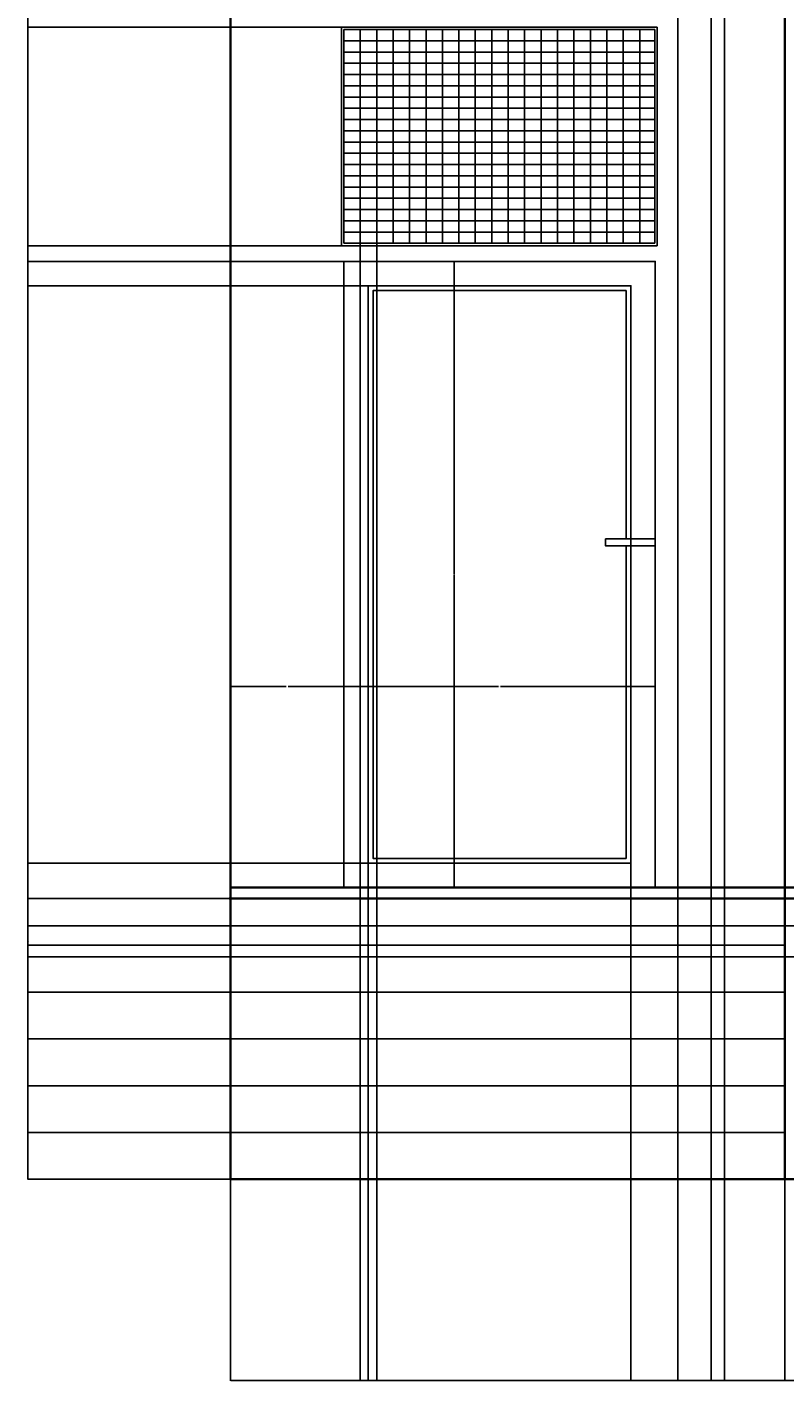
# Model space of a CAD drawing. Units: inches. Extents: x 1231 to 2151, y 481 to 2277.
# Tile 1 of 7: x 1231 to 1542, y 481 to 1038. Entities that reach past the tile are written whole.
import ezdxf

# ---------------------------------------------------------------- set-up
doc = ezdxf.new("R2010")
doc.units = ezdxf.units.IN
doc.header["$MEASUREMENT"] = 0
for name, color, linetype, lineweight in [('A-ANNO-DIMS', 2, 'Continuous', 18), ('A-DOOR', 4, 'Continuous', 25), ('A-ELEV', 7, 'Continuous', 35), ('A-FLOR-STRS', 2, 'Continuous', 25), ('A-GLAZ', 3, 'Continuous', 25)]:
    doc.layers.add(name, color=color, linetype=linetype, lineweight=lineweight)
doc.styles.get("Standard").update_dxf_attribs({"font": 'arial.ttf'})
doc.dimstyles.get("Standard").update_dxf_attribs({"dimtxt": 0.18, "dimasz": 0.18, "dimexe": 0.18, "dimexo": 0.0625, "dimgap": 0.09, "dimtad": 0, "dimtih": 1, "dimtoh": 1, "dimdec": 0, "dimzin": 0, "dimdsep": 46, "dimlunit": 3, "dimtxsty": 'Standard', "dimcen": 0.09, "dimadec": 0, "dimazin": 0, "dimtfac": 1, "dimtdec": 0, "dimtofl": 0, "dimtmove": 0, "dimatfit": 3, "dimfxl": 1, "dimtolj": 1, "dimtzin": 0, "dimarcsym": 0})

# ---------------------------------------------------------------- blocks, each defined once
blk = doc.blocks.new('*D1')
at = {"layer": 'A-ANNO-DIMS', "color": 0, "lineweight": -2, "transparency": 16777216}
for p, q in [((1314.24, 563.63), (1314.24, 480.76)), ((2067.47, 563.63), (2067.47, 480.76)), ((1314.42, 480.94), (1690.47, 480.94)), ((2067.29, 480.94), (1691.25, 480.94))]:
    blk.add_line(p, q, dxfattribs=at)
at = {"layer": 'A-ANNO-DIMS', "color": 0, "transparency": 16777216}
for points in [[(1314.42, 480.97), (1314.42, 480.91), (1314.24, 480.94)], [(2067.29, 480.97), (2067.29, 480.91), (2067.47, 480.94)]]:
    blk.add_solid(points, dxfattribs=at)
at = {"layer": 'Defpoints', "color": 0, "transparency": 16777216}
for p in [(1314.24, 563.69), (2067.47, 563.69), (2067.47, 480.94)]:
    blk.add_point(p, dxfattribs=at)
at = {"layer": 'A-ANNO-DIMS', "color": 0, "transparency": 16777216, "insert": (1690.86, 480.94), "char_height": 0.18, "attachment_point": 5}
blk.add_mtext('\\A1;753.2', dxfattribs=at)
blk = doc.blocks.new('*D2')
at = {"layer": 'A-ANNO-DIMS', "color": 0, "lineweight": -2, "transparency": 16777216}
for p, q in [((1314.18, 2193.78), (1230.78, 2193.78)), ((1230.96, 2193.6), (1230.96, 1378.92)), ((1230.96, 563.87), (1230.96, 1378.55)), ((1314.18, 563.69), (1230.78, 563.69))]:
    blk.add_line(p, q, dxfattribs=at)
at = {"layer": 'A-ANNO-DIMS', "color": 0, "transparency": 16777216}
for points in [[(1230.93, 2193.6), (1230.99, 2193.6), (1230.96, 2193.78)], [(1230.93, 563.87), (1230.99, 563.87), (1230.96, 563.69)]]:
    blk.add_solid(points, dxfattribs=at)
at = {"layer": 'Defpoints', "color": 0, "transparency": 16777216}
for p in [(1230.96, 2193.78), (1314.24, 2193.78), (1314.24, 563.69)]:
    blk.add_point(p, dxfattribs=at)
at = {"layer": 'A-ANNO-DIMS', "color": 0, "transparency": 16777216, "insert": (1230.96, 1378.74), "char_height": 0.18, "attachment_point": 5}
blk.add_mtext('\\A1;1630', dxfattribs=at)
blk = doc.blocks.new('*D29')
at = {"layer": 'A-ANNO-DIMS', "color": 0, "lineweight": -2, "transparency": 16777216}
for p, q in [((1314.24, 683.75), (1314.24, 766.62)), ((1314.42, 766.44), (1337.18, 766.44)), ((1360.73, 766.44), (1337.97, 766.44)), ((1360.91, 683.75), (1360.91, 766.62))]:
    blk.add_line(p, q, dxfattribs=at)
at = {"layer": 'A-ANNO-DIMS', "color": 0, "transparency": 16777216}
for points in [[(1314.42, 766.47), (1314.42, 766.41), (1314.24, 766.44)], [(1360.73, 766.47), (1360.73, 766.41), (1360.91, 766.44)]]:
    blk.add_solid(points, dxfattribs=at)
at = {"layer": 'Defpoints', "color": 0, "transparency": 16777216}
for p in [(1360.91, 766.44), (1314.24, 683.69), (1360.91, 683.69)]:
    blk.add_point(p, dxfattribs=at)
at = {"layer": 'A-ANNO-DIMS', "color": 0, "transparency": 16777216, "insert": (1337.57, 766.44), "char_height": 0.18, "attachment_point": 5}
blk.add_mtext('\\A1;46.67', dxfattribs=at)
blk = doc.blocks.new('*D30')
at = {"layer": 'A-ANNO-DIMS', "color": 0, "lineweight": -2, "transparency": 16777216}
for p, q in [((1360.91, 683.75), (1360.91, 766.62)), ((1361.09, 766.44), (1424.59, 766.44)), ((1488.84, 766.44), (1425.33, 766.44)), ((1489.02, 683.75), (1489.02, 766.62))]:
    blk.add_line(p, q, dxfattribs=at)
at = {"layer": 'A-ANNO-DIMS', "color": 0, "transparency": 16777216}
for points in [[(1361.09, 766.47), (1361.09, 766.41), (1360.91, 766.44)], [(1488.84, 766.47), (1488.84, 766.41), (1489.02, 766.44)]]:
    blk.add_solid(points, dxfattribs=at)
at = {"layer": 'Defpoints', "color": 0, "transparency": 16777216}
for p in [(1489.02, 766.44), (1360.91, 683.69), (1489.02, 683.69)]:
    blk.add_point(p, dxfattribs=at)
at = {"layer": 'A-ANNO-DIMS', "color": 0, "transparency": 16777216, "insert": (1424.96, 766.44), "char_height": 0.18, "attachment_point": 5}
blk.add_mtext('\\A1;128.1', dxfattribs=at)
blk = doc.blocks.new('*D31')
at = {"layer": 'A-ANNO-DIMS', "color": 0, "lineweight": -2, "transparency": 16777216}
for p, q in [((1488.95, 941.31), (1406.09, 941.31)), ((1406.27, 941.13), (1406.27, 812.68)), ((1406.27, 683.87), (1406.27, 812.32)), ((1488.95, 683.69), (1406.09, 683.69))]:
    blk.add_line(p, q, dxfattribs=at)
at = {"layer": 'A-ANNO-DIMS', "color": 0, "transparency": 16777216}
for points in [[(1406.24, 941.13), (1406.3, 941.13), (1406.27, 941.31)], [(1406.24, 683.87), (1406.3, 683.87), (1406.27, 683.69)]]:
    blk.add_solid(points, dxfattribs=at)
at = {"layer": 'Defpoints', "color": 0, "transparency": 16777216}
for p in [(1406.27, 941.31), (1489.02, 941.31), (1489.02, 683.69)]:
    blk.add_point(p, dxfattribs=at)
at = {"layer": 'A-ANNO-DIMS', "color": 0, "transparency": 16777216, "insert": (1406.27, 812.5), "char_height": 0.18, "attachment_point": 5}
blk.add_mtext('\\A1;257.6', dxfattribs=at)
blk = doc.blocks.new('*D37')
at = {"layer": 'A-ANNO-DIMS', "color": 0, "lineweight": -2, "transparency": 16777216}
for p, q in [((1489.79, 947.76), (1230.78, 947.76)), ((1230.96, 947.58), (1230.96, 944.71)), ((1488.95, 941.31), (1230.78, 941.31)), ((1230.96, 941.49), (1230.96, 944.35))]:
    blk.add_line(p, q, dxfattribs=at)
at = {"layer": 'A-ANNO-DIMS', "color": 0, "transparency": 16777216}
for points in [[(1230.93, 947.58), (1230.99, 947.58), (1230.96, 947.76)], [(1230.93, 941.49), (1230.99, 941.49), (1230.96, 941.31)]]:
    blk.add_solid(points, dxfattribs=at)
at = {"layer": 'Defpoints', "color": 0, "transparency": 16777216}
for p in [(1230.96, 947.76), (1489.86, 947.76), (1489.02, 941.31)]:
    blk.add_point(p, dxfattribs=at)
at = {"layer": 'A-ANNO-DIMS', "color": 0, "transparency": 16777216, "insert": (1230.96, 944.53), "char_height": 0.18, "attachment_point": 5}
blk.add_mtext('\\A1;6.453', dxfattribs=at)
blk = doc.blocks.new('*D38')
at = {"layer": 'A-ANNO-DIMS', "color": 0, "lineweight": -2, "transparency": 16777216}
for p, q in [((1489.79, 1037.69), (1230.78, 1037.69)), ((1230.96, 1037.51), (1230.96, 992.91)), ((1230.96, 947.94), (1230.96, 992.54)), ((1489.79, 947.76), (1230.78, 947.76))]:
    blk.add_line(p, q, dxfattribs=at)
at = {"layer": 'A-ANNO-DIMS', "color": 0, "transparency": 16777216}
for points in [[(1230.93, 1037.51), (1230.99, 1037.51), (1230.96, 1037.69)], [(1230.93, 947.94), (1230.99, 947.94), (1230.96, 947.76)]]:
    blk.add_solid(points, dxfattribs=at)
at = {"layer": 'Defpoints', "color": 0, "transparency": 16777216}
for p in [(1230.96, 1037.69), (1489.86, 1037.69), (1489.86, 947.76)]:
    blk.add_point(p, dxfattribs=at)
at = {"layer": 'A-ANNO-DIMS', "color": 0, "transparency": 16777216, "insert": (1230.96, 992.72), "char_height": 0.18, "attachment_point": 5}
blk.add_mtext('\\A1;89.93', dxfattribs=at)
blk = doc.blocks.new('*D39')
at = {"layer": 'A-ANNO-DIMS', "color": 0, "lineweight": -2, "transparency": 16777216}
for p, q in [((1367.67, 948.7), (1367.67, 480.76)), ((1374.43, 948.7), (1374.43, 480.76)), ((1367.85, 480.94), (1370.66, 480.94)), ((1374.25, 480.94), (1371.44, 480.94))]:
    blk.add_line(p, q, dxfattribs=at)
at = {"layer": 'A-ANNO-DIMS', "color": 0, "transparency": 16777216}
for points in [[(1367.85, 480.97), (1367.85, 480.91), (1367.67, 480.94)], [(1374.25, 480.97), (1374.25, 480.91), (1374.43, 480.94)]]:
    blk.add_solid(points, dxfattribs=at)
at = {"layer": 'Defpoints', "color": 0, "transparency": 16777216}
for p in [(1367.67, 948.76), (1374.43, 948.76), (1374.43, 480.94)]:
    blk.add_point(p, dxfattribs=at)
at = {"layer": 'A-ANNO-DIMS', "color": 0, "transparency": 16777216, "insert": (1371.05, 480.94), "char_height": 0.18, "attachment_point": 5}
blk.add_mtext('\\A1;6.762', dxfattribs=at)
blk = doc.blocks.new('*D40')
at = {"layer": 'A-ANNO-DIMS', "color": 0, "lineweight": -2, "transparency": 16777216}
for p, q in [((1370.91, 931.24), (1370.91, 480.76)), ((1479.02, 931.24), (1479.02, 480.76)), ((1371.09, 480.94), (1424.59, 480.94)), ((1478.84, 480.94), (1425.33, 480.94))]:
    blk.add_line(p, q, dxfattribs=at)
at = {"layer": 'A-ANNO-DIMS', "color": 0, "transparency": 16777216}
for points in [[(1371.09, 480.97), (1371.09, 480.91), (1370.91, 480.94)], [(1478.84, 480.97), (1478.84, 480.91), (1479.02, 480.94)]]:
    blk.add_solid(points, dxfattribs=at)
at = {"layer": 'Defpoints', "color": 0, "transparency": 16777216}
for p in [(1370.91, 931.31), (1479.02, 931.31), (1479.02, 480.94)]:
    blk.add_point(p, dxfattribs=at)
at = {"layer": 'A-ANNO-DIMS', "color": 0, "transparency": 16777216, "insert": (1424.96, 480.94), "char_height": 0.18, "attachment_point": 5}
blk.add_mtext('\\A1;108.1', dxfattribs=at)
blk = doc.blocks.new('*D41')
at = {"layer": 'A-ANNO-DIMS', "color": 0, "lineweight": -2, "transparency": 16777216}
for p, q in [((1370.84, 931.31), (1230.78, 931.31)), ((1230.96, 931.13), (1230.96, 812.68)), ((1230.96, 693.87), (1230.96, 812.32)), ((1370.84, 693.69), (1230.78, 693.69))]:
    blk.add_line(p, q, dxfattribs=at)
at = {"layer": 'A-ANNO-DIMS', "color": 0, "transparency": 16777216}
for points in [[(1230.93, 931.13), (1230.99, 931.13), (1230.96, 931.31)], [(1230.93, 693.87), (1230.99, 693.87), (1230.96, 693.69)]]:
    blk.add_solid(points, dxfattribs=at)
at = {"layer": 'Defpoints', "color": 0, "transparency": 16777216}
for p in [(1230.96, 931.31), (1370.91, 931.31), (1370.91, 693.69)]:
    blk.add_point(p, dxfattribs=at)
at = {"layer": 'A-ANNO-DIMS', "color": 0, "transparency": 16777216, "insert": (1230.96, 812.5), "char_height": 0.18, "attachment_point": 5}
blk.add_mtext('\\A1;237.6', dxfattribs=at)
blk = doc.blocks.new('*D42')
at = {"layer": 'A-ANNO-DIMS', "color": 0, "lineweight": -2, "transparency": 16777216}
for p, q in [((1314.09, 582.95), (1230.78, 582.95)), ((1230.96, 582.77), (1230.96, 573.5)), ((1230.96, 563.87), (1230.96, 573.14)), ((1314.18, 563.69), (1230.78, 563.69))]:
    blk.add_line(p, q, dxfattribs=at)
at = {"layer": 'A-ANNO-DIMS', "color": 0, "transparency": 16777216}
for points in [[(1230.93, 582.77), (1230.99, 582.77), (1230.96, 582.95)], [(1230.93, 563.87), (1230.99, 563.87), (1230.96, 563.69)]]:
    blk.add_solid(points, dxfattribs=at)
at = {"layer": 'Defpoints', "color": 0, "transparency": 16777216}
for p in [(1230.96, 582.95), (1314.15, 582.95), (1314.24, 563.69)]:
    blk.add_point(p, dxfattribs=at)
at = {"layer": 'A-ANNO-DIMS', "color": 0, "transparency": 16777216, "insert": (1230.96, 573.32), "char_height": 0.18, "attachment_point": 5}
blk.add_mtext('\\A1;19.26', dxfattribs=at)
blk = doc.blocks.new('*D43')
at = {"layer": 'A-ANNO-DIMS', "color": 0, "lineweight": -2, "transparency": 16777216}
for p, q in [((1314, 602.21), (1230.78, 602.21)), ((1230.96, 602.03), (1230.96, 592.76)), ((1230.96, 583.13), (1230.96, 592.4)), ((1314.09, 582.95), (1230.78, 582.95))]:
    blk.add_line(p, q, dxfattribs=at)
at = {"layer": 'A-ANNO-DIMS', "color": 0, "transparency": 16777216}
for points in [[(1230.93, 602.03), (1230.99, 602.03), (1230.96, 602.21)], [(1230.93, 583.13), (1230.99, 583.13), (1230.96, 582.95)]]:
    blk.add_solid(points, dxfattribs=at)
at = {"layer": 'Defpoints', "color": 0, "transparency": 16777216}
for p in [(1230.96, 602.21), (1314.06, 602.21), (1314.15, 582.95)]:
    blk.add_point(p, dxfattribs=at)
at = {"layer": 'A-ANNO-DIMS', "color": 0, "transparency": 16777216, "insert": (1230.96, 592.58), "char_height": 0.18, "attachment_point": 5}
blk.add_mtext('\\A1;19.26', dxfattribs=at)
blk = doc.blocks.new('*D44')
at = {"layer": 'A-ANNO-DIMS', "color": 0, "lineweight": -2, "transparency": 16777216}
for p, q in [((1313.91, 621.47), (1230.78, 621.47)), ((1230.96, 621.29), (1230.96, 612.02)), ((1230.96, 602.39), (1230.96, 611.66)), ((1314, 602.21), (1230.78, 602.21))]:
    blk.add_line(p, q, dxfattribs=at)
at = {"layer": 'A-ANNO-DIMS', "color": 0, "transparency": 16777216}
for points in [[(1230.93, 621.29), (1230.99, 621.29), (1230.96, 621.47)], [(1230.93, 602.39), (1230.99, 602.39), (1230.96, 602.21)]]:
    blk.add_solid(points, dxfattribs=at)
at = {"layer": 'Defpoints', "color": 0, "transparency": 16777216}
for p in [(1230.96, 621.47), (1313.98, 621.47), (1314.06, 602.21)]:
    blk.add_point(p, dxfattribs=at)
at = {"layer": 'A-ANNO-DIMS', "color": 0, "transparency": 16777216, "insert": (1230.96, 611.84), "char_height": 0.18, "attachment_point": 5}
blk.add_mtext('\\A1;19.26', dxfattribs=at)
blk = doc.blocks.new('*D45')
at = {"layer": 'A-ANNO-DIMS', "color": 0, "lineweight": -2, "transparency": 16777216}
for p, q in [((1313.83, 640.73), (1230.78, 640.73)), ((1230.96, 640.55), (1230.96, 631.28)), ((1230.96, 621.65), (1230.96, 630.91)), ((1313.91, 621.47), (1230.78, 621.47))]:
    blk.add_line(p, q, dxfattribs=at)
at = {"layer": 'A-ANNO-DIMS', "color": 0, "transparency": 16777216}
for points in [[(1230.93, 640.55), (1230.99, 640.55), (1230.96, 640.73)], [(1230.93, 621.65), (1230.99, 621.65), (1230.96, 621.47)]]:
    blk.add_solid(points, dxfattribs=at)
at = {"layer": 'Defpoints', "color": 0, "transparency": 16777216}
for p in [(1230.96, 640.73), (1313.89, 640.73), (1313.98, 621.47)]:
    blk.add_point(p, dxfattribs=at)
at = {"layer": 'A-ANNO-DIMS', "color": 0, "transparency": 16777216, "insert": (1230.96, 631.1), "char_height": 0.18, "attachment_point": 5}
blk.add_mtext('\\A1;19.26', dxfattribs=at)
blk = doc.blocks.new('*D46')
at = {"layer": 'A-ANNO-DIMS', "color": 0, "lineweight": -2, "transparency": 16777216}
for p, q in [((1313.74, 659.98), (1230.78, 659.98)), ((1230.96, 659.8), (1230.96, 650.54)), ((1230.96, 640.91), (1230.96, 650.17)), ((1313.83, 640.73), (1230.78, 640.73))]:
    blk.add_line(p, q, dxfattribs=at)
at = {"layer": 'A-ANNO-DIMS', "color": 0, "transparency": 16777216}
for points in [[(1230.93, 659.8), (1230.99, 659.8), (1230.96, 659.98)], [(1230.93, 640.91), (1230.99, 640.91), (1230.96, 640.73)]]:
    blk.add_solid(points, dxfattribs=at)
at = {"layer": 'Defpoints', "color": 0, "transparency": 16777216}
for p in [(1230.96, 659.98), (1313.8, 659.98), (1313.89, 640.73)]:
    blk.add_point(p, dxfattribs=at)
at = {"layer": 'A-ANNO-DIMS', "color": 0, "transparency": 16777216, "insert": (1230.96, 650.36), "char_height": 0.18, "attachment_point": 5}
blk.add_mtext('\\A1;19.26', dxfattribs=at)
blk = doc.blocks.new('*D47')
at = {"layer": 'A-ANNO-DIMS', "color": 0, "lineweight": -2, "transparency": 16777216}
for p, q in [((1313.65, 679.24), (1230.78, 679.24)), ((1230.96, 679.06), (1230.96, 669.8)), ((1230.96, 660.16), (1230.96, 669.43)), ((1313.74, 659.98), (1230.78, 659.98))]:
    blk.add_line(p, q, dxfattribs=at)
at = {"layer": 'A-ANNO-DIMS', "color": 0, "transparency": 16777216}
for points in [[(1230.93, 679.06), (1230.99, 679.06), (1230.96, 679.24)], [(1230.93, 660.16), (1230.99, 660.16), (1230.96, 659.98)]]:
    blk.add_solid(points, dxfattribs=at)
at = {"layer": 'Defpoints', "color": 0, "transparency": 16777216}
for p in [(1230.96, 679.24), (1313.71, 679.24), (1313.8, 659.98)]:
    blk.add_point(p, dxfattribs=at)
at = {"layer": 'A-ANNO-DIMS', "color": 0, "transparency": 16777216, "insert": (1230.96, 669.61), "char_height": 0.18, "attachment_point": 5}
blk.add_mtext('\\A1;19.26', dxfattribs=at)
blk = doc.blocks.new('*D48')
at = {"layer": 'A-ANNO-DIMS', "color": 0, "lineweight": -2, "transparency": 16777216}
for p, q in [((1314.24, 563.63), (1314.24, 480.76)), ((1542.38, 563.63), (1542.38, 480.76)), ((1314.42, 480.94), (1427.84, 480.94)), ((1542.2, 480.94), (1428.77, 480.94))]:
    blk.add_line(p, q, dxfattribs=at)
at = {"layer": 'A-ANNO-DIMS', "color": 0, "transparency": 16777216}
for points in [[(1314.42, 480.97), (1314.42, 480.91), (1314.24, 480.94)], [(1542.2, 480.97), (1542.2, 480.91), (1542.38, 480.94)]]:
    blk.add_solid(points, dxfattribs=at)
at = {"layer": 'Defpoints', "color": 0, "transparency": 16777216}
for p in [(1314.24, 563.69), (1542.38, 563.69), (1542.38, 480.94)]:
    blk.add_point(p, dxfattribs=at)
at = {"layer": 'A-ANNO-DIMS', "color": 0, "transparency": 16777216, "insert": (1428.31, 480.94), "char_height": 0.18, "attachment_point": 5}
blk.add_mtext('\\A1;228.13', dxfattribs=at)
blk = doc.blocks.new('*D55')
at = {"layer": 'A-ANNO-DIMS', "color": 0, "lineweight": -2, "transparency": 16777216}
for p, q in [((1558.65, 668.02), (1230.78, 668.02)), ((1230.96, 667.84), (1230.96, 661.8)), ((1230.96, 655.39), (1230.96, 661.43)), ((1558.65, 655.21), (1230.78, 655.21))]:
    blk.add_line(p, q, dxfattribs=at)
at = {"layer": 'A-ANNO-DIMS', "color": 0, "transparency": 16777216}
for points in [[(1230.93, 667.84), (1230.99, 667.84), (1230.96, 668.02)], [(1230.93, 655.39), (1230.99, 655.39), (1230.96, 655.21)]]:
    blk.add_solid(points, dxfattribs=at)
at = {"layer": 'Defpoints', "color": 0, "transparency": 16777216}
for p in [(1230.96, 668.02), (1558.72, 668.02), (1558.72, 655.21)]:
    blk.add_point(p, dxfattribs=at)
at = {"layer": 'A-ANNO-DIMS', "color": 0, "transparency": 16777216, "insert": (1230.96, 661.62), "char_height": 0.18, "attachment_point": 5}
blk.add_mtext('\\A1;12.808', dxfattribs=at)
blk = doc.blocks.new('*D66')
at = {"layer": 'A-ANNO-DIMS', "color": 0, "lineweight": -2, "transparency": 16777216}
for p, q in [((1314.24, 1170.27), (1314.24, 480.76)), ((1498.31, 1170.27), (1498.31, 480.76)), ((1314.42, 480.94), (1405.82, 480.94)), ((1498.13, 480.94), (1406.73, 480.94))]:
    blk.add_line(p, q, dxfattribs=at)
at = {"layer": 'A-ANNO-DIMS', "color": 0, "transparency": 16777216}
for points in [[(1314.42, 480.97), (1314.42, 480.91), (1314.24, 480.94)], [(1498.13, 480.97), (1498.13, 480.91), (1498.31, 480.94)]]:
    blk.add_solid(points, dxfattribs=at)
at = {"layer": 'Defpoints', "color": 0, "transparency": 16777216}
for p in [(1314.24, 1170.34), (1498.31, 1170.34), (1498.31, 480.94)]:
    blk.add_point(p, dxfattribs=at)
at = {"layer": 'A-ANNO-DIMS', "color": 0, "transparency": 16777216, "insert": (1406.28, 480.94), "char_height": 0.18, "attachment_point": 5}
blk.add_mtext('\\A1;184.07', dxfattribs=at)
blk = doc.blocks.new('*D68')
at = {"layer": 'A-ANNO-DIMS', "color": 0, "lineweight": -2, "transparency": 16777216}
for p, q in [((1314.24, 1085.65), (1314.24, 480.76)), ((1512.01, 1085.65), (1512.01, 480.76)), ((1314.42, 480.94), (1412.67, 480.94)), ((1511.83, 480.94), (1413.58, 480.94))]:
    blk.add_line(p, q, dxfattribs=at)
at = {"layer": 'A-ANNO-DIMS', "color": 0, "transparency": 16777216}
for points in [[(1314.42, 480.97), (1314.42, 480.91), (1314.24, 480.94)], [(1511.83, 480.97), (1511.83, 480.91), (1512.01, 480.94)]]:
    blk.add_solid(points, dxfattribs=at)
at = {"layer": 'Defpoints', "color": 0, "transparency": 16777216}
for p in [(1314.24, 1085.71), (1512.01, 1085.71), (1512.01, 480.94)]:
    blk.add_point(p, dxfattribs=at)
at = {"layer": 'A-ANNO-DIMS', "color": 0, "transparency": 16777216, "insert": (1413.13, 480.94), "char_height": 0.18, "attachment_point": 5}
blk.add_mtext('\\A1;197.77', dxfattribs=at)
blk = doc.blocks.new('*D69')
at = {"layer": 'A-ANNO-DIMS', "color": 0, "lineweight": -2, "transparency": 16777216}
for p, q in [((1512.01, 1085.65), (1512.01, 480.76)), ((1937.57, 1085.65), (1937.57, 480.76)), ((1512.19, 480.94), (1724.39, 480.94)), ((1937.39, 480.94), (1725.19, 480.94))]:
    blk.add_line(p, q, dxfattribs=at)
at = {"layer": 'A-ANNO-DIMS', "color": 0, "transparency": 16777216}
for points in [[(1512.19, 480.97), (1512.19, 480.91), (1512.01, 480.94)], [(1937.39, 480.97), (1937.39, 480.91), (1937.57, 480.94)]]:
    blk.add_solid(points, dxfattribs=at)
at = {"layer": 'Defpoints', "color": 0, "transparency": 16777216}
for p in [(1512.01, 1085.71), (1937.57, 1085.71), (1937.57, 480.94)]:
    blk.add_point(p, dxfattribs=at)
at = {"layer": 'A-ANNO-DIMS', "color": 0, "transparency": 16777216, "insert": (1724.79, 480.94), "char_height": 0.18, "attachment_point": 5}
blk.add_mtext('\\A1;425.6', dxfattribs=at)
blk = doc.blocks.new('*D70')
at = {"layer": 'A-ANNO-DIMS', "color": 0, "lineweight": -2, "transparency": 16777216}
for p, q in [((1517.5, 1116.1), (1517.5, 480.76)), ((1512.01, 1101.52), (1512.01, 480.76)), ((1512.19, 480.94), (1514.36, 480.94)), ((1517.32, 480.94), (1515.15, 480.94))]:
    blk.add_line(p, q, dxfattribs=at)
at = {"layer": 'A-ANNO-DIMS', "color": 0, "transparency": 16777216}
for points in [[(1512.19, 480.97), (1512.19, 480.91), (1512.01, 480.94)], [(1517.32, 480.97), (1517.32, 480.91), (1517.5, 480.94)]]:
    blk.add_solid(points, dxfattribs=at)
at = {"layer": 'Defpoints', "color": 0, "transparency": 16777216}
for p in [(1517.5, 1116.16), (1512.01, 1101.58), (1517.5, 480.94)]:
    blk.add_point(p, dxfattribs=at)
at = {"layer": 'A-ANNO-DIMS', "color": 0, "transparency": 16777216, "insert": (1514.76, 480.94), "char_height": 0.18, "attachment_point": 5}
blk.add_mtext('\\A1;5.493', dxfattribs=at)
blk = doc.blocks.new('*D71')
at = {"layer": 'A-ANNO-DIMS', "color": 0, "lineweight": -2, "transparency": 16777216}
for p, q in [((1517.5, 1116.1), (1517.5, 480.76)), ((1595.89, 1116.1), (1595.89, 480.76)), ((1517.68, 480.94), (1556.31, 480.94)), ((1595.71, 480.94), (1557.09, 480.94))]:
    blk.add_line(p, q, dxfattribs=at)
at = {"layer": 'A-ANNO-DIMS', "color": 0, "transparency": 16777216}
for points in [[(1517.68, 480.97), (1517.68, 480.91), (1517.5, 480.94)], [(1595.71, 480.97), (1595.71, 480.91), (1595.89, 480.94)]]:
    blk.add_solid(points, dxfattribs=at)
at = {"layer": 'Defpoints', "color": 0, "transparency": 16777216}
for p in [(1517.5, 1116.16), (1595.89, 1116.16), (1595.89, 480.94)]:
    blk.add_point(p, dxfattribs=at)
at = {"layer": 'A-ANNO-DIMS', "color": 0, "transparency": 16777216, "insert": (1556.7, 480.94), "char_height": 0.18, "attachment_point": 5}
blk.add_mtext('\\A1;78.39', dxfattribs=at)

msp = doc.modelspace()

# ---------------------------------------------------------------- linework, layer by layer
at = {"layer": 'A-DOOR'}
for points in [[(1360.9075, 683.6912), (1489.0152, 683.6912), (1489.0152, 941.3064), (1360.9075, 941.3064)], [(1468.5425, 827.174), (1489.0152, 827.174), (1489.0152, 824.3452), (1468.5425, 824.3452)]]:
    msp.add_lwpolyline(points, close=True, dxfattribs=at)
for points in [[(1479.0152, 827.174), (1479.0152, 931.3064), (1370.9075, 931.3064), (1370.9075, 693.6912), (1479.0152, 693.6912), (1479.0152, 824.3452)], [(1477.0152, 827.174), (1477.0152, 929.3064), (1372.9075, 929.3064), (1372.9075, 695.6912), (1477.0152, 695.6912), (1477.0152, 824.3452)]]:
    msp.add_lwpolyline(points, dxfattribs=at)
at = {"layer": 'A-ELEV'}
for p, q in [((1314.2408, 1926.2862), (1314.2408, 563.6912)), ((1542.3752, 1043.6912), (1542.3752, 563.6912)), ((1314.2408, 683.6912), (2067.6855, 683.6912)), ((1313.7129, 679.2431), (2067.6855, 679.2431)), ((1313.7129, 679.2431), (2067.6855, 679.2431)), ((1314.2408, 563.6912), (2067.6855, 563.6912))]:
    msp.add_line(p, q, dxfattribs=at)
at = {"layer": 'A-FLOR-STRS'}
for p, q in [((1313.8009, 659.9845), (1542.3752, 659.9845)), ((1313.8889, 640.7258), (1542.3752, 640.7258)), ((1313.9768, 621.4672), (1542.3752, 621.4672)), ((1314.0648, 602.2085), (1542.3752, 602.2085)), ((1314.1528, 582.9499), (1542.3752, 582.9499))]:
    msp.add_line(p, q, dxfattribs=at)
at = {"layer": 'A-GLAZ'}
for p, q in [((1359.9075, 1037.6872), (1489.8565, 1037.6872)), ((1359.9075, 1037.6872), (1359.9075, 947.7593)), ((1488.8565, 1036.6872), (1360.9075, 1036.6872)), ((1360.9075, 1036.6872), (1360.9075, 948.7593)), ((1360.9075, 1036.6872), (1488.8565, 1036.6872)), ((1367.6698, 1036.6872), (1367.6698, 948.7593)), ((1374.4321, 1036.6872), (1374.4321, 948.7593)), ((1381.1944, 1036.6872), (1381.1944, 948.7593)), ((1387.9567, 1036.6872), (1387.9567, 948.7593)), ((1394.719, 1036.6872), (1394.719, 948.7593)), ((1401.4813, 1036.6872), (1401.4813, 948.7593)), ((1408.2436, 1036.6872), (1408.2436, 948.7593)), ((1415.0059, 1036.6872), (1415.0059, 948.7593)), ((1421.7682, 1036.6872), (1421.7682, 948.7593)), ((1428.5305, 1036.6872), (1428.5305, 948.7593)), ((1435.2928, 1036.6872), (1435.2928, 948.7593)), ((1442.0552, 1036.6872), (1442.0552, 948.7593)), ((1448.8175, 1036.6872), (1448.8175, 948.7593)), ((1455.5798, 1036.6872), (1455.5798, 948.7593)), ((1462.3421, 1036.6872), (1462.3421, 948.7593)), ((1469.1044, 1036.6872), (1469.1044, 948.7593)), ((1475.8667, 1036.6872), (1475.8667, 948.7593)), ((1482.629, 1036.6872), (1482.629, 948.7593)), ((1488.8565, 948.7593), (1488.8565, 1036.6872)), ((1489.8565, 947.7593), (1489.8565, 1037.6872)), ((1360.9075, 1032.0594), (1488.8565, 1032.0594)), ((1360.9075, 1027.4316), (1488.8565, 1027.4316)), ((1360.9075, 1022.8038), (1488.8565, 1022.8038)), ((1360.9075, 1018.1761), (1488.8565, 1018.1761)), ((1360.9075, 1013.5483), (1488.8565, 1013.5483)), ((1360.9075, 1008.9205), (1488.8565, 1008.9205)), ((1360.9075, 1004.2927), (1488.8565, 1004.2927)), ((1360.9075, 999.6649), (1488.8565, 999.6649)), ((1360.9075, 995.0371), (1488.8565, 995.0371)), ((1360.9075, 990.4094), (1488.8565, 990.4094)), ((1360.9075, 985.7816), (1488.8565, 985.7816)), ((1360.9075, 981.1538), (1488.8565, 981.1538)), ((1360.9075, 976.526), (1488.8565, 976.526)), ((1360.9075, 971.8982), (1488.8565, 971.8982)), ((1360.9075, 967.2704), (1488.8565, 967.2704)), ((1360.9075, 962.6427), (1488.8565, 962.6427)), ((1360.9075, 958.0149), (1488.8565, 958.0149)), ((1360.9075, 953.3871), (1488.8565, 953.3871)), ((1359.9075, 947.7593), (1489.8565, 947.7593)), ((1360.9075, 948.7593), (1488.8565, 948.7593))]:
    msp.add_line(p, q, dxfattribs=at)

# ---------------------------------------------------------------- dimensions: what is measured, and where the dimension line sits
at = {"layer": 'A-ANNO-DIMS'}
for base, p1, p2, override, picture, middle in [((1230.9629, 2193.7789), (1314.2408, 563.6912), (1314.2408, 2193.7789), {"dimdec": 0, "dimlfac": 1, "dimrnd": 0, "dimzin": 0, "dimdsep": 46, "dimlunit": 2}, '*D2', (1230.9629, 1378.7351)), ((1230.9629, 1037.6872), (1489.8565, 947.7593), (1489.8565, 1037.6872), {"dimdec": 2, "dimlfac": 1, "dimrnd": 0, "dimzin": 0, "dimdsep": 46, "dimlunit": 2}, '*D38', (1230.9629, 992.7232)), ((1230.9629, 947.7593), (1489.0152, 941.3064), (1489.8565, 947.7593), {"dimdec": 3, "dimlfac": 1, "dimrnd": 0, "dimzin": 0, "dimdsep": 46, "dimlunit": 2}, '*D37', (1230.9629, 944.5329)), ((1406.2652, 941.3064), (1489.0152, 683.6912), (1489.0152, 941.3064), {"dimdec": 1, "dimlfac": 1, "dimrnd": 0, "dimzin": 0, "dimdsep": 46, "dimlunit": 2}, '*D31', (1406.2652, 812.4988)), ((1230.9629, 931.3064), (1370.9075, 693.6912), (1370.9075, 931.3064), {"dimdec": 1, "dimlfac": 1, "dimrnd": 0, "dimzin": 0, "dimdsep": 46, "dimlunit": 2}, '*D41', (1230.9629, 812.4988)), ((1230.9629, 679.2431), (1313.8009, 659.9845), (1313.7129, 679.2431), {"dimdec": 2, "dimlfac": 1, "dimrnd": 0, "dimzin": 0, "dimdsep": 46, "dimlunit": 2}, '*D47', (1230.9629, 669.6138)), ((1230.9629, 668.0208), (1558.7166, 655.2124), (1558.7166, 668.0208), {"dimdec": 3, "dimlfac": 1, "dimrnd": 0, "dimzin": 0, "dimdsep": 46, "dimlunit": 2}, '*D55', (1230.9629, 661.6166)), ((1230.9629, 659.9845), (1313.8889, 640.7258), (1313.8009, 659.9845), {"dimdec": 2, "dimlfac": 1, "dimrnd": 0, "dimzin": 0, "dimdsep": 46, "dimlunit": 2}, '*D46', (1230.9629, 650.3552)), ((1230.9629, 640.7258), (1313.9768, 621.4672), (1313.8889, 640.7258), {"dimdec": 2, "dimlfac": 1, "dimrnd": 0, "dimzin": 0, "dimdsep": 46, "dimlunit": 2}, '*D45', (1230.9629, 631.0965)), ((1230.9629, 621.4672), (1314.0648, 602.2085), (1313.9768, 621.4672), {"dimdec": 2, "dimlfac": 1, "dimrnd": 0, "dimzin": 0, "dimdsep": 46, "dimlunit": 2}, '*D44', (1230.9629, 611.8379)), ((1230.9629, 602.2085), (1314.1528, 582.9499), (1314.0648, 602.2085), {"dimdec": 2, "dimlfac": 1, "dimrnd": 0, "dimzin": 0, "dimdsep": 46, "dimlunit": 2}, '*D43', (1230.9629, 592.5792)), ((1230.9629, 582.9499), (1314.2408, 563.6912), (1314.1528, 582.9499), {"dimdec": 2, "dimlfac": 1, "dimrnd": 0, "dimzin": 0, "dimdsep": 46, "dimlunit": 2}, '*D42', (1230.9629, 573.3206))]:
    dim = msp.add_linear_dim(base=base, p1=p1, p2=p2, angle=90, dimstyle='Standard', override=override, dxfattribs=at)
    dim.commit()
    dim.dimension.update_dxf_attribs({"geometry": picture, "text_midpoint": middle})
for base, p1, p2, override, picture, middle in [((1498.3132, 480.9412), (1314.2408, 1170.3352), (1498.3132, 1170.3352), {"dimdec": 2, "dimlfac": 1, "dimrnd": 0, "dimzin": 0, "dimdsep": 46, "dimlunit": 2}, '*D66', (1406.277, 480.9412)), ((1517.5039, 480.9412), (1512.0105, 1101.5825), (1517.5039, 1116.1584), {"dimdec": 3, "dimlfac": 1, "dimrnd": 0, "dimzin": 0, "dimdsep": 46, "dimlunit": 2}, '*D70', (1514.7572, 480.9412)), ((1595.8928, 480.9412), (1517.5039, 1116.1584), (1595.8928, 1116.1584), {"dimdec": 2, "dimlfac": 1, "dimrnd": 0, "dimzin": 0, "dimdsep": 46, "dimlunit": 2}, '*D71', (1556.6984, 480.9412)), ((1512.0105, 480.9412), (1314.2408, 1085.7079), (1512.0105, 1085.7079), {"dimdec": 2, "dimlfac": 1, "dimrnd": 0, "dimzin": 0, "dimdsep": 46, "dimlunit": 2}, '*D68', (1413.1257, 480.9412)), ((1937.5725, 480.9412), (1512.0105, 1085.7079), (1937.5725, 1085.7079), {"dimdec": 1, "dimlfac": 1, "dimrnd": 0, "dimzin": 0, "dimdsep": 46, "dimlunit": 2}, '*D69', (1724.7915, 480.9412)), ((1374.4321, 480.9412), (1367.6698, 948.7593), (1374.4321, 948.7593), {"dimdec": 3, "dimlfac": 1, "dimrnd": 0, "dimzin": 0, "dimdsep": 46, "dimlunit": 2}, '*D39', (1371.0509, 480.9412)), ((1479.0152, 480.9412), (1370.9075, 931.3064), (1479.0152, 931.3064), {"dimdec": 1, "dimlfac": 1, "dimrnd": 0, "dimzin": 0, "dimdsep": 46, "dimlunit": 2}, '*D40', (1424.9613, 480.9412)), ((1360.9075, 766.4412), (1314.2408, 683.6912), (1360.9075, 683.6912), {"dimdec": 2, "dimlfac": 1, "dimrnd": 0, "dimzin": 0, "dimdsep": 46, "dimlunit": 2}, '*D29', (1337.5741, 766.4412)), ((1489.0152, 766.4412), (1360.9075, 683.6912), (1489.0152, 683.6912), {"dimdec": 1, "dimlfac": 1, "dimrnd": 0, "dimzin": 0, "dimdsep": 46, "dimlunit": 2}, '*D30', (1424.9613, 766.4412)), ((2067.4747, 480.9412), (1314.2408, 563.6912), (2067.4747, 563.6912), {"dimdec": 1, "dimlfac": 1, "dimrnd": 0, "dimzin": 0, "dimdsep": 46, "dimlunit": 2}, '*D1', (1690.8578, 480.9412)), ((1542.3752, 480.9412), (1314.2408, 563.6912), (1542.3752, 563.6912), {"dimdec": 2, "dimlfac": 1, "dimrnd": 0, "dimzin": 0, "dimdsep": 46, "dimlunit": 2}, '*D48', (1428.308, 480.9412))]:
    dim = msp.add_linear_dim(base=base, p1=p1, p2=p2, dimstyle='Standard', override=override, dxfattribs=at)
    dim.commit()
    dim.dimension.update_dxf_attribs({"geometry": picture, "text_midpoint": middle})

doc.saveas('drawing.dxf')
